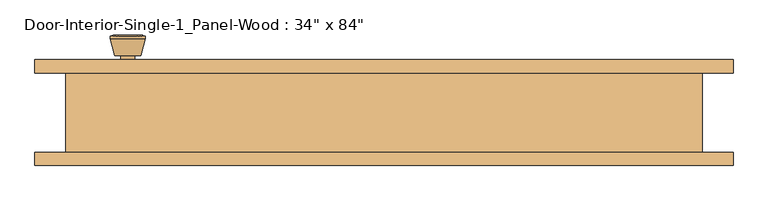
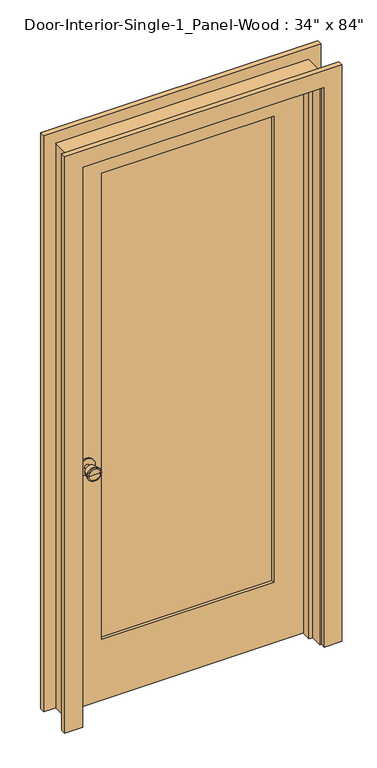
"""IFC4 building model written with IfcOpenShell, lengths in millimetres: door geometry."""

from ifc_helpers import new_model, si_unit, point, frame, frame_2d, origin, place, context, project, spatial, polyline, circle_curve, trimmed, segment, composite_curve, outline, extrude, faceted_brep, source, transform, mapped, element, save
from ifc_brep_helpers import plane_surface, cylinder_surface, revolved_surface, advanced_brep


def door_51292941(model_context):
    return source(origin(), model_context, "Body", "SolidModel", [
        advanced_brep(
        [(-368.3, 13.05, 914.4), (-358.3, 13.05, 914.4), (-378.3, 13.05, 914.4), (-347.8241324, -35.95, 914.4), (-368.3, -35.95, 914.4), (-388.7758676, -35.95, 914.4), (-343.3, -34.1221319, 914.4), (-393.3, -34.1221319, 914.4), (-343.3, -30.6584537, 914.4), (-393.3, -30.6584537, 914.4), (-349.663764, -5.95, 914.4), (-386.936236, -5.95, 914.4), (-358.3, -5.95, 914.4), (-378.3, -5.95, 914.4)],
        [
            (0, 1),
            (1, 2, circle_curve(frame((-368.3, 13.05, 914.4), z_axis=(0.0, 1.0, 0.0), x_axis=(-1.0, 0.0, 0.0)), 10.0)),
            (2, 0),
            (2, 1, circle_curve(frame((-368.3, 13.05, 914.4), z_axis=(0.0, 1.0, 0.0), x_axis=(-1.0, 0.0, 0.0)), 10.0)),
            (3, 4),
            (4, 5),
            (5, 3, circle_curve(frame((-368.3, -35.95, 914.4), z_axis=(0.0, -1.0, 0.0), x_axis=(-1.0, 0.0, 0.0)), 20.4758676)),
            (3, 5, circle_curve(frame((-368.3, -35.95, 914.4), z_axis=(0.0, -1.0, 0.0), x_axis=(-1.0, 0.0, 0.0)), 20.4758676)),
            (6, 3),
            (5, 7),
            (7, 6, circle_curve(frame((-368.3, -34.1221319, 914.4), z_axis=(0.0, -1.0, 0.0), x_axis=(-1.0, 0.0, 0.0)), 25.0)),
            (6, 7, circle_curve(frame((-368.3, -34.1221319, 914.4), z_axis=(0.0, -1.0, 0.0), x_axis=(-1.0, 0.0, 0.0)), 25.0)),
            (8, 6),
            (7, 9),
            (9, 8, circle_curve(frame((-368.3, -30.6584537, 914.4), z_axis=(0.0, -1.0, 0.0), x_axis=(-1.0, 0.0, 0.0)), 25.0)),
            (8, 9, circle_curve(frame((-368.3, -30.6584537, 914.4), z_axis=(0.0, -1.0, 0.0), x_axis=(-1.0, 0.0, 0.0)), 25.0)),
            (10, 8),
            (9, 11),
            (11, 10, circle_curve(frame((-368.3, -5.95, 914.4), z_axis=(0.0, -1.0, 0.0), x_axis=(-1.0, 0.0, 0.0)), 18.636236)),
            (10, 11, circle_curve(frame((-368.3, -5.95, 914.4), z_axis=(0.0, -1.0, 0.0), x_axis=(-1.0, 0.0, 0.0)), 18.636236)),
            (12, 10),
            (11, 13),
            (13, 12, circle_curve(frame((-368.3, -5.95, 914.4), z_axis=(0.0, -1.0, 0.0), x_axis=(-1.0, 0.0, 0.0)), 10.0)),
            (12, 13, circle_curve(frame((-368.3, -5.95, 914.4), z_axis=(0.0, -1.0, 0.0), x_axis=(-1.0, 0.0, 0.0)), 10.0)),
            (1, 12),
            (13, 2),
        ],
        [
            plane_surface(frame((-368.3, 13.05, 914.4), z_axis=(0.0, 1.0, 0.0), x_axis=(-1.0, 0.0, 0.0))),
            plane_surface(frame((-368.3, -35.95, 914.4), z_axis=(0.0, -1.0, 0.0), x_axis=(-1.0, 0.0, 0.0))),
            revolved_surface(polyline([(-388.7758676, -35.95, 914.4), (-393.3, -34.1221319, 914.4)]), (-368.3, 13.05, 914.4), (0.0, 1.0, 0.0)),
            cylinder_surface(frame((-368.3, 13.05, 914.4), z_axis=(0.0, 1.0, 0.0), x_axis=(-1.0, 0.0, 0.0)), 25.0),
            revolved_surface(polyline([(-393.3, -30.6584537, 914.4), (-386.936236, -5.95, 914.4)]), (-368.3, 13.05, 914.4), (0.0, 1.0, 0.0)),
            plane_surface(frame((-368.3, -5.95, 914.4), z_axis=(0.0, 1.0, 0.0), x_axis=(-1.0, 0.0, 0.0))),
            cylinder_surface(frame((-368.3, 13.05, 914.4), z_axis=(0.0, 1.0, 0.0), x_axis=(-1.0, 0.0, 0.0)), 10.0),
        ],
        [
            (0, [[1, 2, 3]]),
            (0, [[-3, 4, -1]]),
            (1, [[5, 6, 7]]),
            (1, [[-6, -5, 8]]),
            (2, [[9, -7, 10, 11]]),
            (2, [[-10, -8, -9, 12]]),
            (3, [[13, -11, 14, 15]]),
            (3, [[-14, -12, -13, 16]]),
            (4, [[17, -15, 18, 19]]),
            (4, [[-18, -16, -17, 20]]),
            (5, [[21, -19, 22, 23]]),
            (5, [[-22, -20, -21, 24]]),
            (6, [[25, -23, 26, -2]]),
            (6, [[-26, -24, -25, -4]]),
        ],
    ),
        extrude(outline(composite_curve([segment(trimmed(circle_curve(frame_2d((914.4, -368.3)), 30.0), [point((914.4, -398.3))], [point((914.4, -338.3))], False, "CARTESIAN"), True, "CONTINUOUS"), segment(trimmed(circle_curve(frame_2d((914.4, -368.3)), 30.0), [point((914.4, -338.3))], [point((914.4, -398.3))], False, "CARTESIAN"), True, "CONTINUOUS")], self_intersect=False)), frame((0.0, 13.05, 0.0), z_axis=(0.0, 1.0, 0.0), x_axis=(0.0, 0.0, 1.0)), (0.0, 0.0, 1.0), 6.0),
        advanced_brep(
        [(-368.3, 59.975, 914.4), (-378.3, 59.975, 914.4), (-358.3, 59.975, 914.4), (-347.8241324, 108.975, 914.4), (-388.7758676, 108.975, 914.4), (-368.3, 108.975, 914.4), (-343.3, 107.1471319, 914.4), (-393.3, 107.1471319, 914.4), (-343.3, 103.6834537, 914.4), (-393.3, 103.6834537, 914.4), (-349.663764, 78.975, 914.4), (-386.936236, 78.975, 914.4), (-358.3, 78.975, 914.4), (-378.3, 78.975, 914.4)],
        [
            (0, 1),
            (1, 2, circle_curve(frame((-368.3, 59.975, 914.4), z_axis=(0.0, -1.0, 0.0), x_axis=(-1.0, 0.0, 0.0)), 10.0)),
            (2, 0),
            (2, 1, circle_curve(frame((-368.3, 59.975, 914.4), z_axis=(0.0, -1.0, 0.0), x_axis=(-1.0, 0.0, 0.0)), 10.0)),
            (3, 4, circle_curve(frame((-368.3, 108.975, 914.4), z_axis=(0.0, 1.0, 0.0), x_axis=(-1.0, 0.0, 0.0)), 20.4758676)),
            (4, 5),
            (5, 3),
            (4, 3, circle_curve(frame((-368.3, 108.975, 914.4), z_axis=(0.0, 1.0, 0.0), x_axis=(-1.0, 0.0, 0.0)), 20.4758676)),
            (6, 7, circle_curve(frame((-368.3, 107.1471319, 914.4), z_axis=(0.0, 1.0, 0.0), x_axis=(-1.0, 0.0, 0.0)), 25.0)),
            (7, 4),
            (3, 6),
            (7, 6, circle_curve(frame((-368.3, 107.1471319, 914.4), z_axis=(0.0, 1.0, 0.0), x_axis=(-1.0, 0.0, 0.0)), 25.0)),
            (8, 9, circle_curve(frame((-368.3, 103.6834537, 914.4), z_axis=(0.0, 1.0, 0.0), x_axis=(-1.0, 0.0, 0.0)), 25.0)),
            (9, 7),
            (6, 8),
            (9, 8, circle_curve(frame((-368.3, 103.6834537, 914.4), z_axis=(0.0, 1.0, 0.0), x_axis=(-1.0, 0.0, 0.0)), 25.0)),
            (10, 11, circle_curve(frame((-368.3, 78.975, 914.4), z_axis=(0.0, 1.0, 0.0), x_axis=(-1.0, 0.0, 0.0)), 18.636236)),
            (11, 9),
            (8, 10),
            (11, 10, circle_curve(frame((-368.3, 78.975, 914.4), z_axis=(0.0, 1.0, 0.0), x_axis=(-1.0, 0.0, 0.0)), 18.636236)),
            (12, 13, circle_curve(frame((-368.3, 78.975, 914.4), z_axis=(0.0, 1.0, 0.0), x_axis=(-1.0, 0.0, 0.0)), 10.0)),
            (13, 11),
            (10, 12),
            (13, 12, circle_curve(frame((-368.3, 78.975, 914.4), z_axis=(0.0, 1.0, 0.0), x_axis=(-1.0, 0.0, 0.0)), 10.0)),
            (1, 13),
            (12, 2),
        ],
        [
            plane_surface(frame((-368.3, 59.975, 914.4), z_axis=(0.0, -1.0, 0.0), x_axis=(-1.0, 0.0, 0.0))),
            plane_surface(frame((-368.3, 108.975, 914.4), z_axis=(0.0, 1.0, 0.0), x_axis=(-1.0, 0.0, 0.0))),
            revolved_surface(polyline([(-388.7758676, 108.975, 914.4), (-393.3, 107.1471319, 914.4)]), (-368.3, 59.975, 914.4), (0.0, -1.0, 0.0)),
            cylinder_surface(frame((-368.3, 59.975, 914.4), z_axis=(0.0, -1.0, 0.0), x_axis=(-1.0, 0.0, 0.0)), 25.0),
            revolved_surface(polyline([(-393.3, 103.6834537, 914.4), (-386.936236, 78.975, 914.4)]), (-368.3, 59.975, 914.4), (0.0, -1.0, 0.0)),
            plane_surface(frame((-368.3, 78.975, 914.4), z_axis=(0.0, -1.0, 0.0), x_axis=(-1.0, 0.0, 0.0))),
            cylinder_surface(frame((-368.3, 59.975, 914.4), z_axis=(0.0, -1.0, 0.0), x_axis=(-1.0, 0.0, 0.0)), 10.0),
        ],
        [
            (0, [[1, 2, 3]]),
            (0, [[-3, 4, -1]]),
            (1, [[5, 6, 7]]),
            (1, [[8, -7, -6]]),
            (2, [[9, 10, -5, 11]]),
            (2, [[12, -11, -8, -10]]),
            (3, [[13, 14, -9, 15]]),
            (3, [[16, -15, -12, -14]]),
            (4, [[17, 18, -13, 19]]),
            (4, [[20, -19, -16, -18]]),
            (5, [[21, 22, -17, 23]]),
            (5, [[24, -23, -20, -22]]),
            (6, [[-2, 25, -21, 26]]),
            (6, [[-4, -26, -24, -25]]),
        ],
    ),
        extrude(outline(composite_curve([segment(trimmed(circle_curve(frame_2d((914.4, -368.3)), 30.0), [point((914.4, -398.3))], [point((914.4, -338.3))], False, "CARTESIAN"), True, "CONTINUOUS"), segment(trimmed(circle_curve(frame_2d((914.4, -368.3)), 30.0), [point((914.4, -338.3))], [point((914.4, -398.3))], False, "CARTESIAN"), True, "CONTINUOUS")], self_intersect=False)), frame((0.0, 53.975, 0.0), z_axis=(0.0, 1.0, 0.0), x_axis=(0.0, 0.0, 1.0)), (0.0, 0.0, 1.0), 6.0),
        faceted_brep([(457.2, 53.975, 0.0), (457.2, -60.325, 0.0), (431.8, -60.325, 0.0), (431.8, -15.875, 0.0), (419.1, -15.875, 0.0), (419.1, 19.05, 0.0), (431.8, 19.05, 0.0), (431.8, 53.975, 0.0), (457.2, 53.975, 2159.0), (457.2, -60.325, 2159.0), (-457.2, -60.325, 2159.0), (-457.2, -60.325, 0.0), (-431.8, -60.325, 0.0), (-431.8, -60.325, 2133.6), (431.8, -60.325, 2133.6), (431.8, -15.875, 2133.6), (-431.8, -15.875, 2133.6), (-431.8, -15.875, 0.0), (-419.1, -15.875, 0.0), (-419.1, -15.875, 2120.9), (419.1, -15.875, 2120.9), (419.1, 19.05, 2120.9), (-419.1, 19.05, 2120.9), (-419.1, 19.05, 0.0), (-431.8, 19.05, 0.0), (-431.8, 19.05, 2133.6), (431.8, 19.05, 2133.6), (431.8, 53.975, 2133.6), (-431.8, 53.975, 2133.6), (-431.8, 53.975, 0.0), (-457.2, 53.975, 0.0), (-457.2, 53.975, 2159.0)], [[[0, 1, 2, 3, 4, 5, 6, 7]], [[1, 0, 8, 9]], [[2, 1, 9, 10, 11, 12, 13, 14]], [[3, 2, 14, 15]], [[4, 3, 15, 16, 17, 18, 19, 20]], [[5, 4, 20, 21]], [[6, 5, 21, 22, 23, 24, 25, 26]], [[7, 6, 26, 27]], [[0, 7, 27, 28, 29, 30, 31, 8]], [[9, 8, 31, 10]], [[15, 14, 13, 16]], [[21, 20, 19, 22]], [[27, 26, 25, 28]], [[30, 29, 24, 23, 18, 17, 12, 11]], [[10, 31, 30, 11]], [[16, 13, 12, 17]], [[22, 19, 18, 23]], [[28, 25, 24, 29]]]),
        extrude(outline(polyline([(2133.6, -431.8), (0.0, -431.8), (0.0, 431.8), (2133.6, 431.8), (2133.6, -431.8)]), holes=[polyline([(2014.5375, -311.15), (2014.5375, 311.15), (231.775, 311.15), (231.775, -311.15), (2014.5375, -311.15)])]), frame((0.0, 19.05, 0.0), z_axis=(0.0, 1.0, 0.0), x_axis=(0.0, 0.0, 1.0)), (0.0, 0.0, 1.0), 34.925),
        extrude(outline(polyline([(311.15, 30.6916667), (-311.15, 30.6916667), (-311.15, 42.3333333), (311.15, 42.3333333), (311.15, 30.6916667)])), frame((0.0, 0.0, 231.775), z_axis=(0.0, 0.0, 1.0), x_axis=(1.0, 0.0, 0.0)), (0.0, 0.0, 1.0), 1782.7625),
        extrude(outline(polyline([(0.0, 438.15), (0.0, 501.65), (2203.45, 501.65), (2203.45, -501.65), (0.0, -501.65), (0.0, -438.15), (2139.95, -438.15), (2139.95, 438.15), (0.0, 438.15)])), frame((0.0, 53.975, 0.0), z_axis=(0.0, 1.0, 0.0), x_axis=(0.0, 0.0, 1.0)), (0.0, 0.0, 1.0), 19.05),
        extrude(outline(polyline([(0.0, 438.15), (0.0, 501.65), (2203.45, 501.65), (2203.45, -501.65), (0.0, -501.65), (0.0, -438.15), (2139.95, -438.15), (2139.95, 438.15), (0.0, 438.15)])), frame((0.0, -79.375, 0.0), z_axis=(0.0, 1.0, 0.0), x_axis=(0.0, 0.0, 1.0)), (0.0, 0.0, 1.0), 19.05),
    ])


if __name__ == "__main__":
    model = new_model("IFC4")
    model_context = context("Model", 3, world=origin())
    ifc_project = project(units=[si_unit("LENGTHUNIT", "METRE", prefix="MILLI")], contexts=[model_context])
    site = spatial("IfcSite", under=ifc_project)
    building = spatial("IfcBuilding", under=site)
    placement = place(None, origin())
    door_shape = door_51292941(model_context)
    element("IfcDoor", 1, ObjectType="Door-Interior-Single-1_Panel-Wood : 34\" x 84\"", at=placement, inside=building, context=model_context, shape_type="MappedRepresentation", body=[
        mapped(door_shape, transform((0.0, 0.0, 0.0), x_axis=(1.0, 0.0, 0.0), y_axis=(0.0, 1.0, 0.0), z_axis=(0.0, 0.0, 1.0))),
    ])
    save(model, "model.ifc")

# Revit data of these elements
# Type "Door-Interior-Single-1_Panel-Wood : 34\" x 84\""
#   Type Mark = "9"
#   Assembly Code = "C1020300"
#   Analytic Construction = "Wooden"
#   Top Rail = 0.390625 ft
#   Thickness = 0.114583 ft
#   Thermal Resistance (R) = 2.5876 (h·ft²·°F)/BTU
#   Swing Angle [instance default] = 90.00°
#   Stiles = 0.395833 ft
#   Rough Width = 3 ft
#   Rough Height = 7.083333 ft
#   Height = 7 ft
#   Width = 2.833333 ft
#   Heat Transfer Coefficient (U) = 0.3865 BTU/(h·ft²·°F)
#   Bottom Rail = 0.760417 ft
#   Trim Material = Cherry
#   Panel Material = Cherry
#   Frame Material = Cherry
#   Door Handle Material = Aluminum
#   Visual Light Transmittance = 0
#   Solar Heat Gain Coefficient = 0
#   Wall Closure = (empty or 0)
#   Function = (empty or 0)
# Element 1 (IfcDoor, "Door-Interior-Single-1_Panel-Wood : 34\" x 84\"")
#   Materials on its faces: "Cherry", "Aluminum"
# Materials
#   "Cherry": class "Wood", colour RGB 226 177 128, transparency 0, Description = "Prunus Serotina", Cost = 0
#   "Aluminum": class "Metal", colour RGB 247 247 247, transparency 0, Description = "Aluminum 6061", Cost = 0
